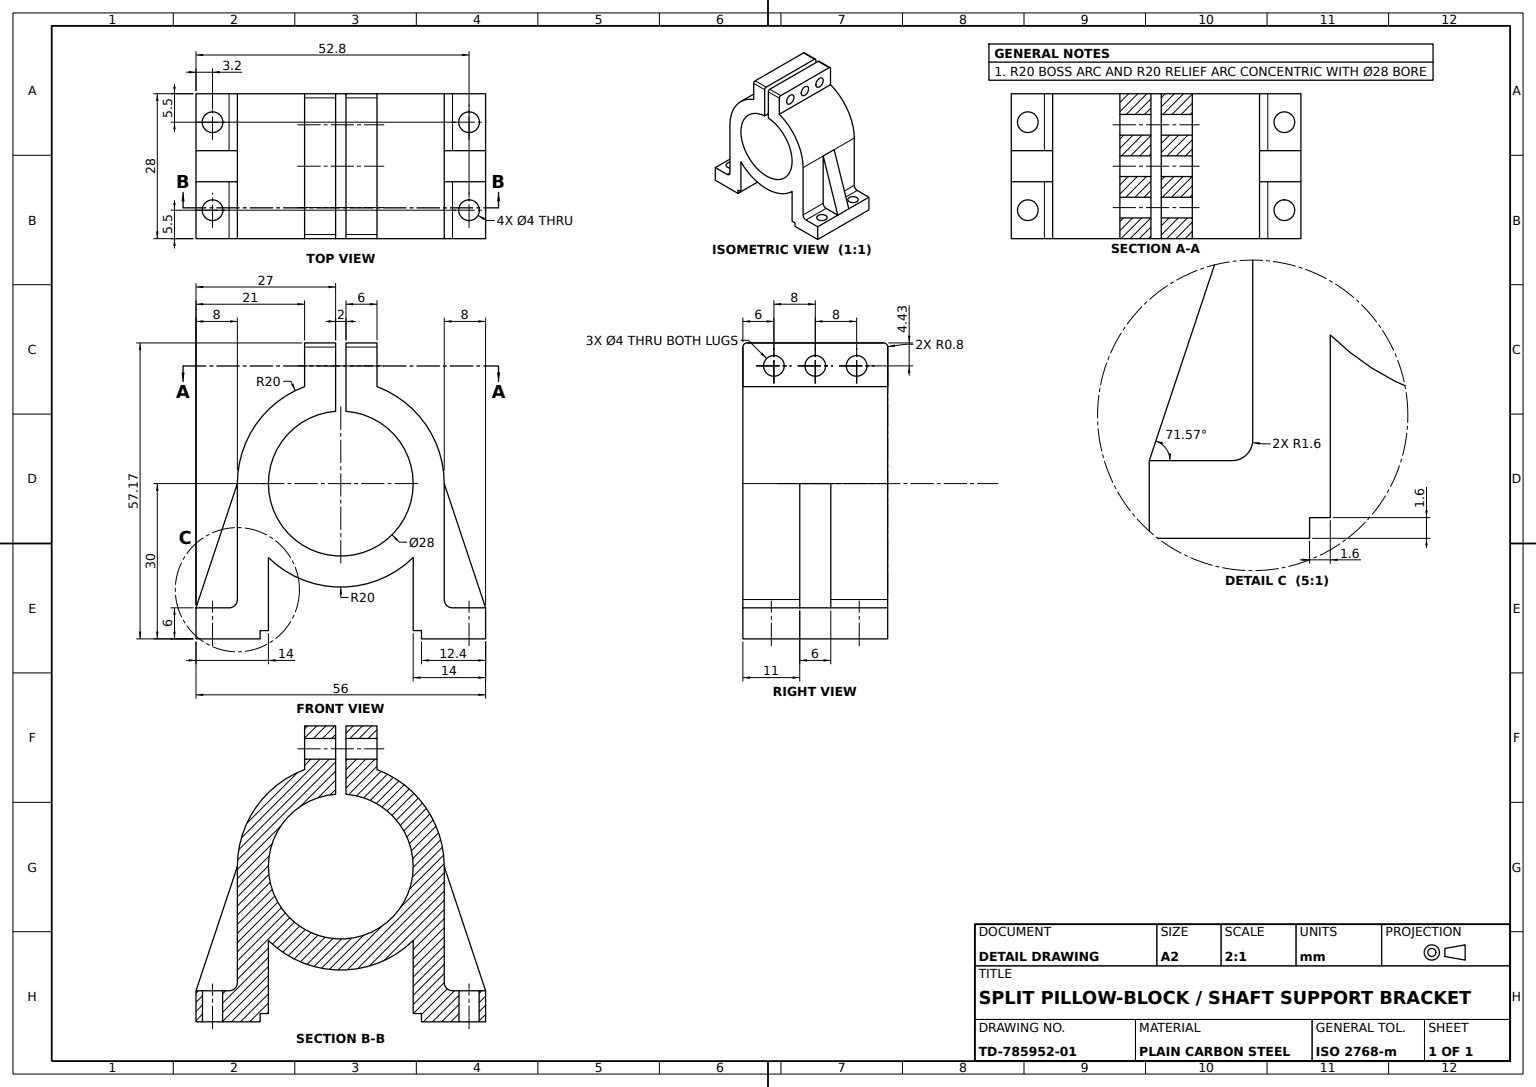
SolidWorks part; units mm, degrees
material "Plain Carbon Steel"
ref_plane "Front Plane" through (0, 0, 0) normal (0, 0, 1) x (1, 0, 0)
ref_plane "Top Plane" through (0, 0, 0) normal (0, 1, 0) x (1, 0, 0)
ref_plane "Right Plane" through (0, 0, 0) normal (1, 0, 0) x (0, 0, -1)
sketch "Clamp Body Profile" plane through (0, 0, 0) normal (0, 0, 1) x (1, 0, 0)
  line L0 (-20, 0) -> (-20, -22.4)
  line L1 (20, 0) -> (20, -22.4)
  line L2 (21.6, -24) -> (28, -24)
  line L3 (28, -24) -> (28, -30)
  line L4 (28, -30) -> (15.6, -30)
  line L5 (15.6, -30) -> (15.6, -28.4)
  line L6 (15.6, -28.4) -> (14, -28.4)
  line L7 (14, -28.4) -> (14, -14.2829)
  line L8 (-21.6, -24) -> (-28, -24)
  line L9 (-28, -24) -> (-28, -30)
  line L10 (-28, -30) -> (-15.6, -30)
  line L11 (-15.6, -30) -> (-15.6, -28.4)
  line L12 (-15.6, -28.4) -> (-14, -28.4)
  line L13 (-14, -28.4) -> (-14, -14.2829)
  line L14 (-1, 19.975) -> (-1, 27.175)
  line L15 (-1, 27.175) -> (-7, 27.175)
  line L16 (-7, 27.175) -> (-7, 18.735)
  line L17 (1, 19.975) -> (1, 27.175)
  line L18 (1, 27.175) -> (7, 27.175)
  line L19 (7, 27.175) -> (7, 18.735)
  line L20 (-1, 19.975) -> (-1, 13.9642)
  line L21 (1, 19.975) -> (1, 13.9642)
  arc A0 (-14, -14.2829) -> (14, -14.2829) centre (0, 0) ccw
  arc A1 (20, 0) -> (7, 18.735) centre (0, 0) ccw
  arc A2 (-7, 18.735) -> (-20, 0) centre (0, 0) ccw
  arc A3 (-1, 13.9642) -> (1, 13.9642) centre (0, 0) ccw
  arc A4 (20, -22.4) -> (21.6, -24) centre (21.6, -22.4) ccw
  arc A5 (-21.6, -24) -> (-20, -22.4) centre (-21.6, -22.4) ccw
  dimension "D1" = 40
  dimension "D2" = 1.6
  dimension "D3" = 1.6
  dimension "D4" = 20
  dimension "D5" = 14
  dimension "D6" = 30
  dimension "D7" = 6
  dimension "D8" = 1.6
  dimension "D9" = 1.6
  dimension "D10" = 14
  dimension "D11" = 30
  dimension "D12" = 28.4
  dimension "D13" = 6.4
  dimension "D14" = 13.2107
  dimension "D15" = 6
  dimension "D16" = 6
  dimension "D17" = 27.175
  dimension "D18" = 14.1171
  dimension "D19" = 1.6
  dimension "D20" = 14.1171
  dimension "D21" = 24
  dimension "D22" = 27.175
  dimension "D23" = 8.44
extrude "Clamp Body" add sketch "Clamp Body Profile" along normal blind 28
sketch "Side Recess A Sketch" plane through (7, 0, 0) normal (1, 0, 0) x (0, 0, -1)
  line L0 (-28, 26.375) -> (-28, 27.175)
  line L1 (-28, 18.735) -> (-28, 27.175) construction
  line L4 (-28, 27.175) -> (-27.2, 27.175)
  arc A0 (-27.2, 27.175) -> (-28, 26.375) centre (-27.2, 26.375) ccw
  dimension "D1" = 0.8
extrude "Side Recess A" cut sketch "Side Recess A Sketch" against normal blind 18
sketch "Side Recess B Sketch" plane through (7, 0, 0) normal (1, 0, 0) x (0, 0, -1)
  line L0 (0, 27.175) -> (0, 26.375)
  line L1 (0, 18.735) -> (0, 27.175) construction
  line L2 (0, 27.175) -> (-0.8, 27.175)
  arc A0 (0, 26.375) -> (-0.8, 27.175) centre (-0.8, 26.375) ccw
  dimension "D1" = 0.8
extrude "Side Recess B" cut sketch "Side Recess B Sketch" against normal blind 18
sketch "Lower Side Boss Sketch" plane through (0, 0, 28) normal (0, 0, 1) x (1, 0, 0)
  line L0 (20, 0) -> (28, -24)
  line L1 (28, -24) -> (21.6, -24)
  line L2 (20, 0) -> (20, -22.4)
  arc A0 (21.6, -24) -> (20, -22.4) centre (21.6, -22.4) cw
  dimension "D1" = 1.6
extrude "Lower Side Boss" add sketch "Lower Side Boss Sketch" against normal blind 28
sketch "Lower Boss Relief A Sketch" plane through (0, 0, 28) normal (0, 0, 1) x (1, 0, 0)
  line L0 (20, 0) -> (28, -24)
  line L1 (28, -24) -> (21.6, -24)
  line L2 (20, -22.4) -> (20, 0)
  arc A0 (21.6, -24) -> (20, -22.4) centre (21.6, -22.4) cw
  dimension "D1" = 1.6
extrude "Lower Boss Relief A" cut sketch "Lower Boss Relief A Sketch" against normal blind 11
sketch "Lower Boss Relief B Sketch" plane through (0, 0, 0) normal (0, 0, -1) x (-1, 0, 0)
  line L2 (-20, 0) -> (-20, -22.4)
  line L3 (-21.6, -24) -> (-28, -24)
  line L4 (-28, -24) -> (-20, 0)
  arc A0 (-21.6, -24) -> (-20, -22.4) centre (-21.6, -22.4) ccw
  dimension "D1" = 1.6
extrude "Lower Boss Relief B" cut sketch "Lower Boss Relief B Sketch" against normal blind 11
sketch "Upper Side Boss Sketch" plane through (0, 0, 0) normal (0, 0, -1) x (-1, 0, 0)
  line L0 (20, 0) -> (28, -24)
  line L1 (28, -24) -> (21.6, -24)
  line L2 (20, -22.4) -> (20, 0)
  arc A0 (21.6, -24) -> (20, -22.4) centre (21.6, -22.4) cw
  dimension "D1" = 1.6
extrude "Upper Side Boss" add sketch "Upper Side Boss Sketch" against normal blind 28
sketch "Upper Boss Relief A Sketch" plane through (0, 0, 0) normal (0, 0, -1) x (-1, 0, 0)
  line L0 (20, 0) -> (20, -22.4)
  line L1 (21.6, -24) -> (28, -24)
  line L2 (28, -24) -> (20, 0)
  arc A0 (20, -22.4) -> (21.6, -24) centre (21.6, -22.4) ccw
  dimension "D1" = 1.6
extrude "Upper Boss Relief A" cut sketch "Upper Boss Relief A Sketch" against normal blind 11
sketch "Upper Boss Relief B Sketch" plane through (0, 0, 28) normal (0, 0, 1) x (1, 0, 0)
  line L0 (-20, 0) -> (-20, -22.4)
  line L1 (-21.6, -24) -> (-28, -24)
  line L2 (-28, -24) -> (-20, 0)
  arc A0 (-20, -22.4) -> (-21.6, -24) centre (-21.6, -22.4) cw
  dimension "D1" = 1.6
extrude "Upper Boss Relief B" cut sketch "Upper Boss Relief B Sketch" against normal blind 11
sketch "Clamp Screw Holes Sketch" plane through (7, 0, 0) normal (1, 0, 0) x (0, 0, -1)
  line L0 (0, 18.735) -> (0, 26.375) construction
  line L1 (-28, 18.735) -> (-28, 26.375) construction
  line L2 (-27.2, 27.175) -> (-0.8, 27.175) construction
  circle A0 centre (-22, 22.7437) radius 2
  circle A1 centre (-14, 22.7437) radius 2
  circle A2 centre (-6, 22.7437) radius 2
  dimension "D1" = 6
  dimension "D4" = 4
  dimension "D2" = 6
  dimension "D3" = 8
  dimension "D5" = 4.4313
extrude "Clamp Screw Holes 3x" cut sketch "Clamp Screw Holes Sketch" against normal blind 20
sketch "Foot Mounting Holes Sketch" plane through (0, -24, 0) normal (0, 1, 0) x (1, 0, 0)
  line L0 (28, -17) -> (20, -17) construction
  line L1 (28, 0) -> (21.6, 0) construction
  line L2 (28, -28) -> (28, -17) construction
  circle A0 centre (24.8, -22.5) radius 2
  circle A1 centre (24.8, -5.5) radius 2
  circle A2 centre (-24.8, -5.5) radius 2
  circle A3 centre (-24.8, -22.5) radius 2
  dimension "D1" = 5.5
  dimension "D2" = 5.5
  dimension "D3" = 4
  dimension "D4" = 3.2
  dimension "D5" = 52.8
extrude "Foot Mounting Holes" cut sketch "Foot Mounting Holes Sketch" against normal blind 20
